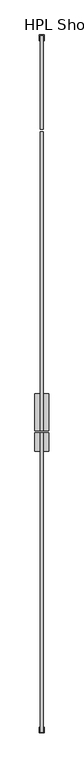
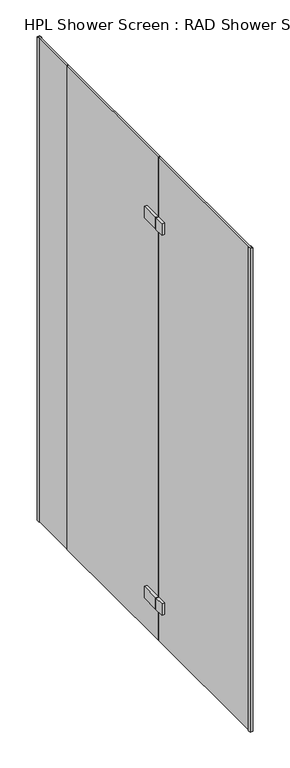
"""IFC4 building model written with IfcOpenShell, lengths in millimetres: flow terminal geometry, HPL Shower Screen : RAD Shower Screen - cut corner."""

from ifc_helpers import new_model, si_unit, frame, origin, origin_with_axes, place, context, project, spatial, polyline, outline, extrude, source, transform, mapped, element, save


def hpl_shower_screen_rad_shower_screen_cut_corner_606f97bc(model_context):
    return source(origin(), model_context, "Body", "SweptSolid", [
        extrude(outline(polyline([(18.1750129, 0.0), (11.8249871, 0.0), (11.8249871, 650.0), (18.1750129, 650.0), (18.1750129, 0.0)])), origin_with_axes(), (0.0, 0.0, 1.0), 2100.0),
        extrude(outline(polyline([(30.0, 0.0), (0.0, 0.0), (0.0, 80.0), (30.0, 80.0), (30.0, 0.0)])), frame((0.0, 0.0, 140.0), z_axis=(0.0, 0.0, 1.0), x_axis=(1.0, 0.0, 0.0)), (0.0, 0.0, 1.0), 50.0),
        extrude(outline(polyline([(30.0, 0.0), (0.0, 0.0), (0.0, 80.0), (30.0, 80.0), (30.0, 0.0)])), frame((0.0, 0.0, 1790.0), z_axis=(0.0, 0.0, 1.0), x_axis=(1.0, 0.0, 0.0)), (0.0, 0.0, 1.0), 50.0),
        extrude(outline(polyline([(11.8249871, -654.6974002), (11.8249871, -4.0), (18.1750129, -4.0), (18.1750129, -654.6974002), (11.8249871, -654.6974002)])), origin_with_axes(), (0.0, 0.0, 1.0), 2100.0),
        extrude(outline(polyline([(0.0, -44.0), (0.0, -4.0), (30.0, -4.0), (30.0, -44.0), (0.0, -44.0)])), frame((0.0, 0.0, 140.0), z_axis=(0.0, 0.0, 1.0), x_axis=(1.0, 0.0, 0.0)), (0.0, 0.0, 1.0), 50.0),
        extrude(outline(polyline([(0.0, -44.0), (0.0, -4.0), (30.0, -4.0), (30.0, -44.0), (0.0, -44.0)])), frame((0.0, 0.0, 1790.0), z_axis=(0.0, 0.0, 1.0), x_axis=(1.0, 0.0, 0.0)), (0.0, 0.0, 1.0), 50.0),
        extrude(outline(polyline([(11.8249871, 858.3333333), (18.1750129, 858.3333333), (18.1750129, 655.0), (11.8249871, 655.0), (11.8249871, 858.3333333)])), origin_with_axes(), (0.0, 0.0, 1.0), 2100.0),
        extrude(outline(polyline([(11.8249871, -654.6974002), (18.1750129, -654.6974002), (18.1750129, -644.1974002), (20.1750129, -644.1974002), (20.1750129, -656.6974002), (9.8249871, -656.6974002), (9.8249871, -644.1974002), (11.8249871, -644.1974002), (11.8249871, -654.6974002)])), origin_with_axes(), (0.0, 0.0, 1.0), 2100.0),
        extrude(outline(polyline([(11.8249871, 858.3333333), (11.8249871, 847.8333333), (9.8249871, 847.8333333), (9.8249871, 860.3333333), (20.1750129, 860.3333333), (20.1750129, 847.8333333), (18.1750129, 847.8333333), (18.1750129, 858.3333333), (11.8249871, 858.3333333)])), origin_with_axes(), (0.0, 0.0, 1.0), 2100.0),
    ])


if __name__ == "__main__":
    model = new_model("IFC4")
    model_context = context("Model", 3, world=origin())
    ifc_project = project(units=[si_unit("LENGTHUNIT", "METRE", prefix="MILLI")], contexts=[model_context])
    site = spatial("IfcSite", under=ifc_project)
    building = spatial("IfcBuilding", under=site)
    placement = place(None, origin())
    hpl_shower_screen_rad_shower_screen_cut_corner_shape = hpl_shower_screen_rad_shower_screen_cut_corner_606f97bc(model_context)
    element("IfcFlowTerminal", 1, ObjectType="HPL Shower Screen : RAD Shower Screen - cut corner", at=placement, inside=building, context=model_context, shape_type="MappedRepresentation", body=[
        mapped(hpl_shower_screen_rad_shower_screen_cut_corner_shape, transform((0.0, 0.0, 0.0), x_axis=(1.0, 0.0, 0.0), y_axis=(0.0, 1.0, 0.0), z_axis=(0.0, 0.0, 1.0))),
    ])
    save(model, "model.ifc")

# Revit data of these elements
# Type "HPL Shower Screen : RAD Shower Screen - cut corner"
#   URL = "http://www.matki.co.uk/"
#   Model = "EPW1150 BESPOKE - 'Eauzone Plus' - left hand recess"
#   Manufacturer = "MATKI"
#   Description = "Shower screen - chamfered fixed panel"
#   Fixed panel width [instance default] = 296 mm
#   End Panel Width [instance default] = 100 mm
#   Door Width = 650 mm
#   Offset = 0 mm
#   Height = 2100 mm
#   Door [instance default] = yes
#   Default Elevation = 0
# Element 1 (IfcFlowTerminal, "HPL Shower Screen : RAD Shower Screen - cut corner")
#   Fixed panel width = 650.697 mm
#   End Panel Width = 203.333 mm
#   Materials on its faces: "Metal Joint", "Aluminum 5052", "Glass"
# Materials
#   "Metal Joint": colour RGB 247 247 247, transparency 0
#   "Aluminum 5052": class "Metal", colour RGB 120 120 120, transparency 0, Description = "Aluminum, strain hardened, magnesium alloy, marine", Cost = 0
#   "Glass": class "Glass", colour RGB 0 128 192, transparency 0.9, Description = "Soda Lime Glass", Cost = 0
